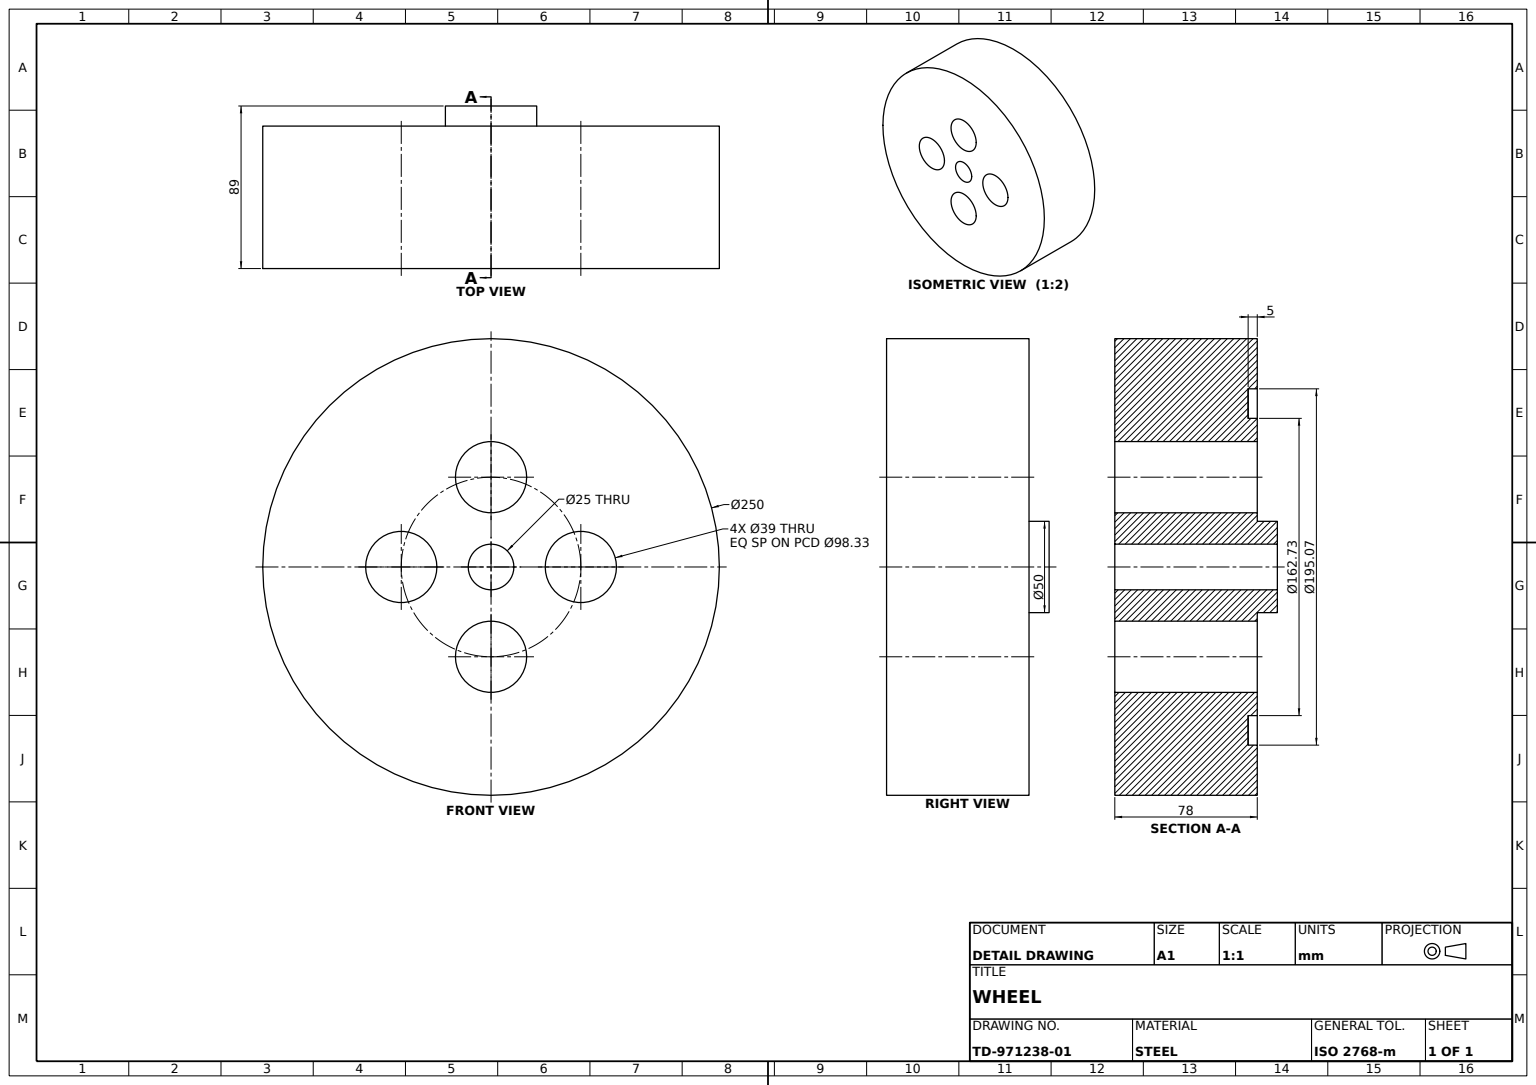
SolidWorks part; units mm, degrees
material "Plain Carbon Steel"
ref_plane "Front Plane" through (0, 0, 0) normal (0, 0, 1) x (1, 0, 0)
ref_plane "Top Plane" through (0, 0, 0) normal (0, 1, 0) x (1, 0, 0)
ref_plane "Right Plane" through (0, 0, 0) normal (1, 0, 0) x (0, 0, -1)
sketch "Wheel Disc Sketch" plane through (0, 0, 0) normal (0, 0, 1) x (1, 0, 0)
  line L0 (0, 342.6651) -> (0, -350.7397) construction
  line L1 (601.5565, 0) -> (-586.4166, 0) construction
  circle A0 centre (0, 0) radius 125
  dimension "D1" = 250
extrude "Wheel Disc Ø250" add sketch "Wheel Disc Sketch" against normal blind 78
sketch "Face Recess Sketch" plane through (0, 0, 0) normal (0, 0, 1) x (1, 0, 0)
  circle A0 centre (0, 0) radius 97.5334
  circle A1 centre (0, 0) radius 81.3671
  dimension "D1" = 162.7343
  dimension "D2" = 195.0668
extrude "Face Recess 5mm" cut sketch "Face Recess Sketch" against normal blind 5
sketch "Lightening Hole 1 Sketch" plane through (0, 0, 0) normal (0, 0, 1) x (1, 0, 0)
  circle A0 centre (0, 0) radius 12.5
  circle A1 centre (0, 0) radius 25
  circle A2 centre (0, 0) radius 49.1626 construction
  circle A3 centre (0, 49.1626) radius 19.5
  circle A4 centre (49.1626, 0) radius 19.5
  circle A5 centre (0, -49.1626) radius 19.5
  circle A6 centre (-49.1626, 0) radius 19.5
  point P16 (0, 0)
  dimension "D1" = 25
  dimension "D2" = 50
  dimension "D3" = 98.3253
  dimension "D4" = 39
  dimension "D5" = 4
extrude "Lightening Hole 1 Ø39" cut sketch "Lightening Hole 1 Sketch" against normal blind 78 contours A3
sketch "Lightening Hole 2 Sketch" plane through (0, 0, 0) normal (0, 0, 1) x (1, 0, 0)
  circle A0 centre (0, 0) radius 49.1626 construction
  circle A2 centre (49.1626, 0) radius 19.5
  dimension "D1" = 39
extrude "Lightening Hole 2 Ø39" cut sketch "Lightening Hole 2 Sketch" against normal blind 78
sketch "Lightening Hole 3 Sketch" plane through (0, 0, 0) normal (0, 0, 1) x (1, 0, 0)
  circle A0 centre (0, 0) radius 49.1626
  circle A1 centre (0, -49.1626) radius 19.5
  dimension "D1" = 39
extrude "Lightening Hole 3 Ø39" cut sketch "Lightening Hole 3 Sketch" against normal blind 78 contours A1
sketch "Lightening Hole 4 Sketch" plane through (0, 0, 0) normal (0, 0, 1) x (1, 0, 0)
  circle A1 centre (-49.1626, 0) radius 19.5
  dimension "D1" = 39
  dimension "D2" = 49.1626
extrude "Lightening Hole 4 Ø39" cut sketch "Lightening Hole 4 Sketch" against normal blind 78
sketch "Hub Boss Sketch" plane through (0, 0, -5) normal (0, 0, 1) x (1, 0, 0)
  circle A0 centre (0, 0) radius 12.5
  circle A1 centre (0, 0) radius 25
  dimension "D1" = 25
  dimension "D2" = 50
extrude "Hub Boss Ø50" add sketch "Hub Boss Sketch" along normal blind 16
sketch "Centre Cut Sketch" plane through (0, 0, 0) normal (0, 0, 1) x (1, 0, 0)
  circle A1 centre (0, 0) radius 12.5
  circle A2 centre (0, 0) radius 12.5
  dimension "D1" = 0
extrude "Centre Cut" cut sketch "Centre Cut Sketch" against normal blind 78
